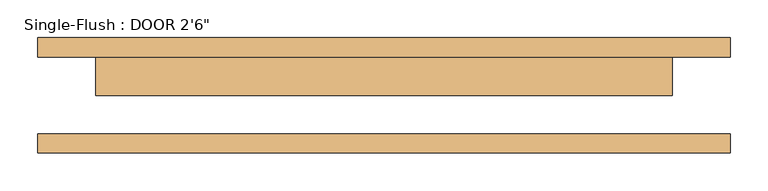
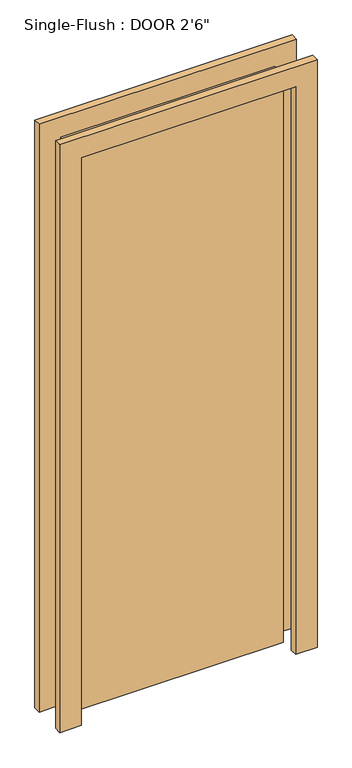
"""IFC4 building model written with IfcOpenShell, lengths in millimetres: door geometry."""

from ifc_helpers import new_model, si_unit, frame, origin, origin_with_axes, place, context, project, spatial, polyline, outline, extrude, source, transform, mapped, element, save


def door_270f2424(model_context):
    return source(origin(), model_context, "Body", "SweptSolid", [
        extrude(outline(polyline([(2209.8, -457.2), (0.0, -457.2), (0.0, -381.0), (2133.6, -381.0), (2133.6, 381.0), (0.0, 381.0), (0.0, 457.2), (2209.8, 457.2), (2209.8, -457.2)])), frame((0.0, 50.8, 0.0), z_axis=(0.0, 1.0, 0.0), x_axis=(0.0, 0.0, 1.0)), (0.0, 0.0, 1.0), 25.4),
        extrude(outline(polyline([(2209.8, 457.2), (2209.8, -457.2), (0.0, -457.2), (0.0, -381.0), (2133.6, -381.0), (2133.6, 381.0), (0.0, 381.0), (0.0, 457.2), (2209.8, 457.2)])), frame((0.0, -76.2, 0.0), z_axis=(0.0, 1.0, 0.0), x_axis=(0.0, 0.0, 1.0)), (0.0, 0.0, 1.0), 25.4),
        extrude(outline(polyline([(381.0, 0.0), (-381.0, 0.0), (-381.0, 50.8), (381.0, 50.8), (381.0, 0.0)])), origin_with_axes(), (0.0, 0.0, 1.0), 2133.6),
    ])


if __name__ == "__main__":
    model = new_model("IFC4")
    model_context = context("Model", 3, world=origin())
    ifc_project = project(units=[si_unit("LENGTHUNIT", "METRE", prefix="MILLI")], contexts=[model_context])
    site = spatial("IfcSite", under=ifc_project)
    building = spatial("IfcBuilding", under=site)
    placement = place(None, origin())
    door_shape = door_270f2424(model_context)
    element("IfcDoor", 1, ObjectType="Single-Flush : DOOR 2'6\"", at=placement, inside=building, context=model_context, shape_type="MappedRepresentation", body=[
        mapped(door_shape, transform((0.0, 0.0, 0.0), x_axis=(1.0, 0.0, 0.0), y_axis=(0.0, 1.0, 0.0), z_axis=(0.0, 0.0, 1.0))),
    ])
    save(model, "model.ifc")

# Revit data of these elements
# Type "Single-Flush : DOOR 2'6\""
#   Type Mark = "9"
#   Construction Type Id = "MDOOR"
#   Assembly Code = "C1020"
#   Analytic Construction = "Metal"
#   Thickness = 0' - 2"
#   Heat Transfer Coefficient (U) = 0.651978 BTU/(h·ft²·°F)
#   Height = 7' - 0"
#   Trim Projection Ext = 0' - 1"
#   Trim Projection Int = 0' - 1"
#   Trim Width = 0' - 3"
#   Width = 2' - 6"
#   Define Thermal Properties by = 1
#   Door Material = Door - Panel
#   Frame Material = Door - Frame
#   Visual Light Transmittance = 0
#   Solar Heat Gain Coefficient = 0
#   Function = (empty or 0)
#   Wall Closure = (empty or 0)
# Element 1 (IfcDoor, "Single-Flush : DOOR 2'6\"")
#   Materials on its faces: "Door - Frame", "Door - Panel"
# Materials
#   "Door - Panel": class "Wood", colour RGB 210 159 95, transparency 0, Cost = 0
#   "Door - Frame": colour RGB 118 70 51, transparency 0, Cost = 0
